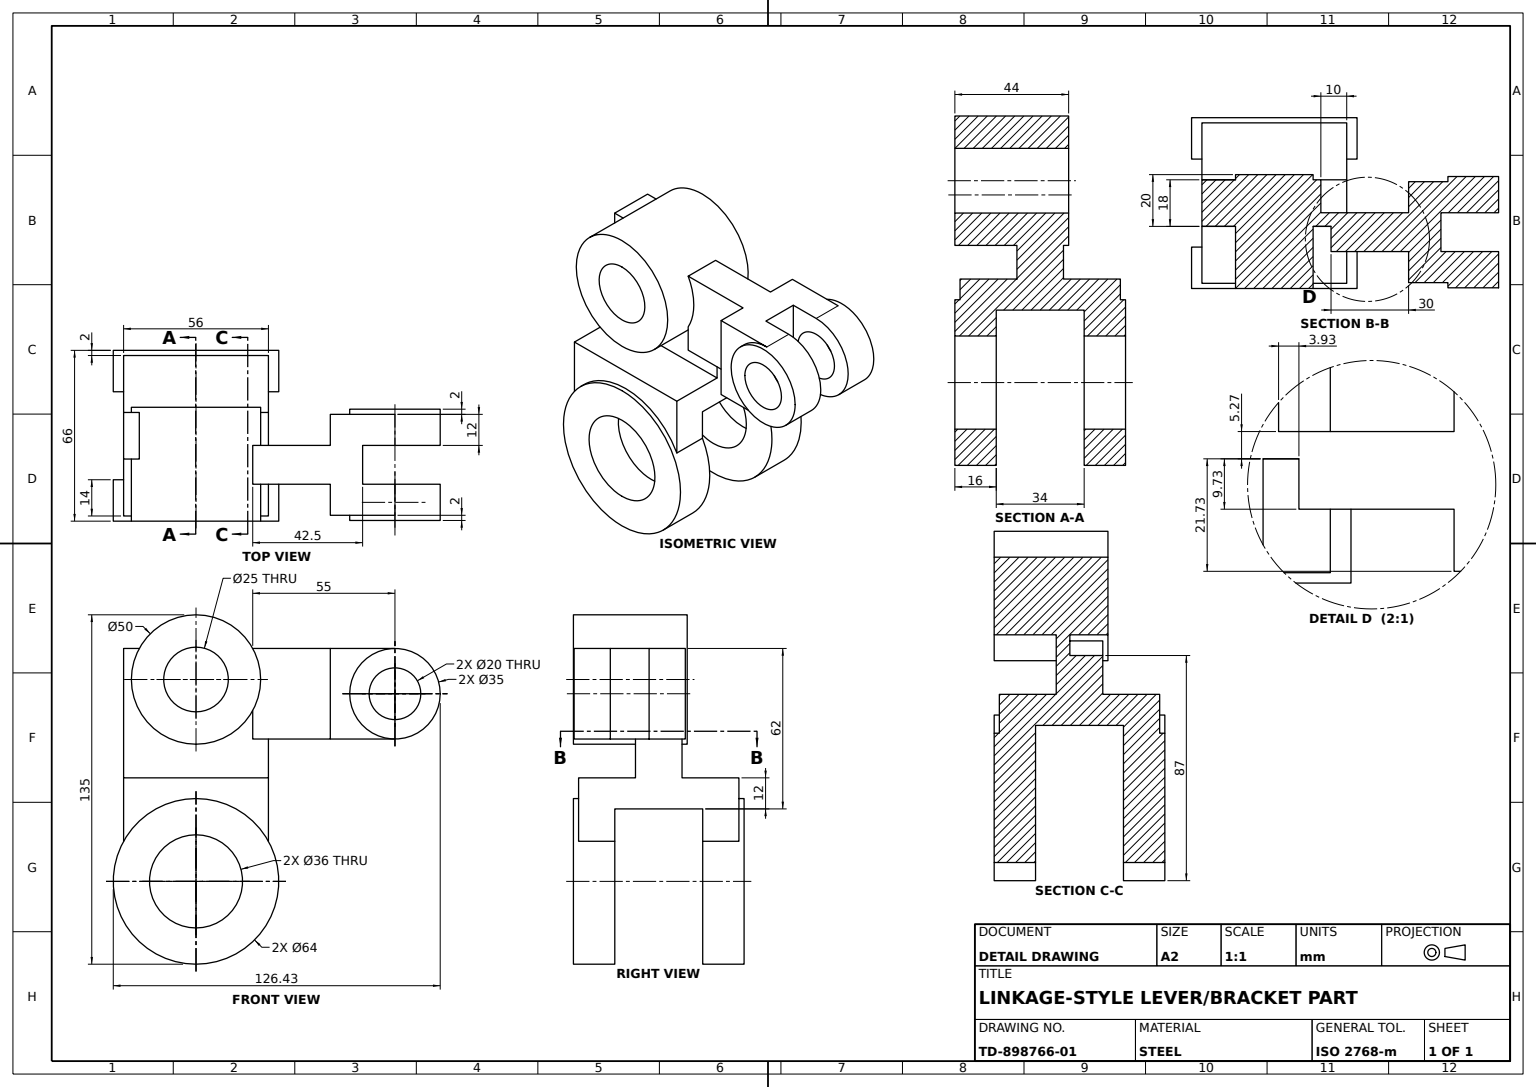
SolidWorks part; units mm, degrees
material "Plain Carbon Steel"
ref_plane "Front Plane" through (0, 0, 0) normal (0, 0, 1) x (1, 0, 0)
ref_plane "Top Plane" through (0, 0, 0) normal (0, 1, 0) x (1, 0, 0)
ref_plane "Right Plane" through (0, 0, 0) normal (1, 0, 0) x (0, 0, -1)
sketch "Bracket Profile Sketch" plane through (0, 0, 0) normal (0, 0, 1) x (1, 0, 0)
  line L0 (0, 0) -> (17, 0)
  line L1 (17, 0) -> (17, -48)
  line L2 (17, -48) -> (31, -48)
  line L3 (0, 0) -> (-17, 0)
  line L4 (-17, 0) -> (-17, -48)
  line L5 (-17, -48) -> (-31, -48)
  line L6 (-31, -48) -> (-31, 12)
  line L7 (-31, 12) -> (-9, 12)
  line L8 (31, 12) -> (31, -48)
  line L9 (0, -48) -> (0, 62) construction
  line L10 (-9, 62) -> (9, 62)
  line L11 (9, 62) -> (9, 12)
  line L12 (-9, 62) -> (-9, 12)
  line L13 (9, 12) -> (31, 12)
  dimension "D1" = 12
  dimension "D2" = 14
  dimension "D3" = 14
  dimension "D4" = 17
  dimension "D5" = 17
  dimension "D6" = 48
  dimension "D7" = 34
  dimension "D8" = 18
  dimension "D9" = 62
extrude "Bracket Body" add sketch "Bracket Profile Sketch" against normal blind 56
sketch "Slot Sketch" plane through (0, 0, 0) normal (0, 0, 1) x (1, 0, 0)
  line L0 (-31, -48) -> (-31, -28)
  line L1 (-31, 12) -> (-31, -48) construction
  line L2 (-31, -28) -> (31, -28)
  line L3 (31, -48) -> (31, 12) construction
  line L4 (31, -28) -> (31, -48)
  line L5 (31, -48) -> (-31, -48)
  dimension "D1" = 20
extrude "Slot Cut" cut sketch "Slot Sketch" against normal through all
sketch "Lug A Sketch" plane through (31, 0, 0) normal (1, 0, 0) x (0, 0, -1)
  line L0 (56, -28) -> (0, -28) construction
  circle A0 centre (28, -28) radius 32
  circle A1 centre (28, -28) radius 18
  dimension "D1" = 36
  dimension "D2" = 64
extrude "Lug A 14mm" add sketch "Lug A Sketch" against normal blind 14
sketch "Spacer A Sketch" plane through (31, 0, 0) normal (1, 0, 0) x (0, 0, -1)
  line L0 (46, -28) -> (10, -28) construction
  circle A0 centre (28, -28) radius 32
  circle A1 centre (28, -28) radius 18
  dimension "D1" = 36
  dimension "D2" = 64
extrude "Spacer A 2mm" add sketch "Spacer A Sketch" along normal blind 2
sketch "Hole A Sketch" plane through (31, 0, 0) normal (1, 0, 0) x (0, 0, -1)
  line L0 (46, -28) -> (10, -28) construction
  circle A0 centre (28, -28) radius 18
  dimension "D1" = 36
extrude "Hole A" cut sketch "Hole A Sketch" against normal through all
sketch "Spacer B Sketch" plane through (-31, 0, 0) normal (-1, 0, 0) x (0, 0, 1)
  circle A0 centre (-28, -28) radius 18
  circle A1 centre (-28, -28) radius 32
  dimension "D1" = 36
  dimension "D2" = 64
extrude "Spacer B 2mm" add sketch "Spacer B Sketch" along normal blind 2
sketch "Lug B Sketch" plane through (-17, 0, 0) normal (1, 0, 0) x (0, 0, -1)
  circle A0 centre (28, -28) radius 18
  circle A1 centre (28, -28) radius 32
  dimension "D1" = 36
  dimension "D2" = 64
extrude "Lug B 14mm" add sketch "Lug B Sketch" against normal blind 14
sketch "Pad Sketch" plane through (-9, 0, 0) normal (-1, 0, 0) x (0, 0, 1)
  line L0 (-28, -60) -> (-28, 50) construction
  line L2 (-56, 62) -> (0, 62) construction
  circle A0 centre (-28, -28) radius 32 construction
  circle A1 centre (-28, 50) radius 25
  circle A2 centre (-28, 50) radius 12.5
  dimension "D1" = 25
  dimension "D2" = 50
  dimension "D3" = 12
extrude "Pad 2mm" add sketch "Pad Sketch" along normal blind 2
sketch "Hub Sketch" plane through (-11, 0, 0) normal (-1, 0, 0) x (0, 0, 1)
  circle A0 centre (-28, 50) radius 12.5
  circle A1 centre (-28, 50) radius 25
  dimension "D1" = 25
  dimension "D2" = 50
extrude "Hub 44mm" add sketch "Hub Sketch" against normal blind 44
sketch "Hub Bore Sketch" plane through (-9, 0, 0) normal (-1, 0, 0) x (0, 0, 1)
  circle A0 centre (-28, 50) radius 12.5
  dimension "D1" = 25
extrude "Hub Bore" cut sketch "Hub Bore Sketch" against normal blind 44
sketch "Arm Profile Sketch" plane through (0, 62, 0) normal (0, 1, 0) x (1, 0, 0)
  line L0 (9, 56) -> (9, 49.9317) construction
  line L1 (9, 49.9317) -> (-9, 49.9317) construction
  line L2 (3.732, 49.9317) -> (3.732, 79.9317)
  line L3 (3.732, 79.9317) -> (-8.268, 79.9317)
  line L4 (-8.268, 79.9317) -> (-8.268, 104.9317)
  line L5 (-8.268, 104.9317) -> (3.732, 104.9317)
  line L6 (3.732, 104.9317) -> (3.732, 92.4317)
  line L7 (3.732, 92.4317) -> (18.732, 92.4317)
  line L8 (18.732, 92.4317) -> (18.732, 104.9317)
  line L9 (18.732, 104.9317) -> (30.732, 104.9317)
  line L10 (30.732, 104.9317) -> (30.732, 79.9317)
  line L11 (30.732, 79.9317) -> (18.732, 79.9317)
  line L12 (18.732, 79.9317) -> (18.732, 49.9317)
  line L13 (3.732, 49.9317) -> (18.732, 49.9317)
  dimension "D1" = 9.732
  dimension "D2" = 21.732
  dimension "D3" = 5.268
  dimension "D4" = 30
  dimension "D5" = 42.5
  dimension "D6" = 55
extrude "Arm 35mm" add sketch "Arm Profile Sketch" against normal blind 35
sketch "Arm Spacer A Sketch" plane through (-8.268, 0, 0) normal (-1, 0, 0) x (0, 0, 1)
  line L0 (-104.9317, 27) -> (-104.9317, 62) construction
  circle A1 centre (-104.9317, 44.5) radius 17.5
  circle A2 centre (-104.9317, 44.5) radius 10
  dimension "D1" = 20
  dimension "D2" = 35
extrude "Arm Spacer A 2mm" add sketch "Arm Spacer A Sketch" along normal blind 2
sketch "Arm Lug Sketch" plane through (-8.268, 0, 0) normal (-1, 0, 0) x (0, 0, 1)
  line L0 (-104.9317, 34.5) -> (-104.9317, 54.5) construction
  circle A0 centre (-104.9317, 44.5) radius 10
  circle A1 centre (-104.9317, 44.5) radius 17.5
  dimension "D1" = 20
  dimension "D2" = 35
extrude "Arm Lug 12mm" add sketch "Arm Lug Sketch" against normal blind 12
sketch "Arm Hole Sketch" plane through (-8.268, 0, 0) normal (-1, 0, 0) x (0, 0, 1)
  line L0 (-104.9317, 34.5) -> (-104.9317, 54.5) construction
  circle A0 centre (-104.9317, 44.5) radius 10
  dimension "D1" = 20
extrude "Arm Hole" cut sketch "Arm Hole Sketch" against normal through all
sketch "Arm Spacer B Sketch" plane through (30.732, 0, 0) normal (1, 0, 0) x (0, 0, -1)
  circle A0 centre (104.9317, 44.5) radius 10
  circle A1 centre (104.9317, 44.5) radius 17.5
  dimension "D1" = 20
  dimension "D2" = 35
extrude "Arm Spacer B 2mm" add sketch "Arm Spacer B Sketch" along normal blind 2
sketch "Arm Eye Sketch" plane through (32.732, 0, 0) normal (1, 0, 0) x (0, 0, -1)
  circle A0 centre (104.9317, 44.5) radius 10
  circle A1 centre (104.9317, 44.5) radius 17.5
  dimension "D1" = 20
  dimension "D2" = 35
extrude "Arm Eye 14mm" add sketch "Arm Eye Sketch" against normal blind 14
sketch "Arm Slot Sketch" plane through (0, 0, -56) normal (0, 0, -1) x (-1, 0, 0)
  line L0 (9, 62) -> (-3.732, 62)
  line L1 (-3.732, 62) -> (-3.732, 27)
  line L2 (-3.732, 27) -> (9, 27)
  line L3 (9, 62) -> (9, 12) construction
  line L4 (9, 27) -> (9, 62)
extrude "Arm Slot 10mm" cut sketch "Arm Slot Sketch" against normal blind 10
sketch "Pin Boss Sketch" plane through (-11, 0, 0) normal (-1, 0, 0) x (0, 0, 1)
  circle A0 centre (-28, 50) radius 25
  dimension "D1" = 50
extrude "Pin Boss 16mm" add sketch "Pin Boss Sketch" against normal blind 16
sketch "Pin Boss Hole Sketch" plane through (-11, 0, 0) normal (-1, 0, 0) x (0, 0, 1)
  circle A0 centre (-28, 50) radius 12.5
  dimension "D1" = 25
extrude "Pin Boss Hole" cut sketch "Pin Boss Hole Sketch" against normal through all
